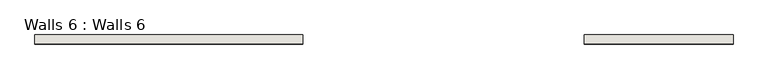
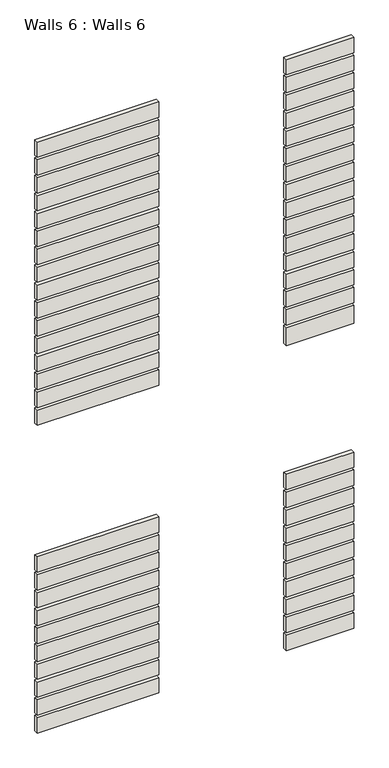
"""IFC4 building model written with IfcOpenShell, lengths in millimetres: wall geometry, Walls 6 : Walls 6."""

from ifc_helpers import new_model, si_unit, frame, origin, place, context, project, spatial, polyline, outline, extrude, source, transform, mapped, element, save


def walls_6_walls_6_f5cc7341(model_context):
    return source(origin(), model_context, "Body", "SweptSolid", [
        extrude(outline(polyline([(142.6430349, 349.9055142), (-2143.3569651, 349.9055142), (-2143.3569651, 426.1055142), (142.6430349, 426.1055142), (142.6430349, 349.9055142)])), frame((0.0, 0.0, 14224.0), z_axis=(0.0, 0.0, 1.0), x_axis=(1.0, 0.0, 0.0)), (0.0, 0.0, 1.0), 304.8),
        extrude(outline(polyline([(142.6430349, 349.9055142), (-2143.3569651, 349.9055142), (-2143.3569651, 426.1055142), (142.6430349, 426.1055142), (142.6430349, 349.9055142)])), frame((0.0, 0.0, 13868.4), z_axis=(0.0, 0.0, 1.0), x_axis=(1.0, 0.0, 0.0)), (0.0, 0.0, 1.0), 304.8),
        extrude(outline(polyline([(142.6430349, 349.9055142), (-2143.3569651, 349.9055142), (-2143.3569651, 426.1055142), (142.6430349, 426.1055142), (142.6430349, 349.9055142)])), frame((0.0, 0.0, 13512.8), z_axis=(0.0, 0.0, 1.0), x_axis=(1.0, 0.0, 0.0)), (0.0, 0.0, 1.0), 304.8),
        extrude(outline(polyline([(142.6430349, 349.9055142), (-2143.3569651, 349.9055142), (-2143.3569651, 426.1055142), (142.6430349, 426.1055142), (142.6430349, 349.9055142)])), frame((0.0, 0.0, 13157.2), z_axis=(0.0, 0.0, 1.0), x_axis=(1.0, 0.0, 0.0)), (0.0, 0.0, 1.0), 304.8),
        extrude(outline(polyline([(142.6430349, 349.9055142), (-2143.3569651, 349.9055142), (-2143.3569651, 426.1055142), (142.6430349, 426.1055142), (142.6430349, 349.9055142)])), frame((0.0, 0.0, 12801.6), z_axis=(0.0, 0.0, 1.0), x_axis=(1.0, 0.0, 0.0)), (0.0, 0.0, 1.0), 304.8),
        extrude(outline(polyline([(142.6430349, 349.9055142), (-2143.3569651, 349.9055142), (-2143.3569651, 426.1055142), (142.6430349, 426.1055142), (142.6430349, 349.9055142)])), frame((0.0, 0.0, 12446.0), z_axis=(0.0, 0.0, 1.0), x_axis=(1.0, 0.0, 0.0)), (0.0, 0.0, 1.0), 304.8),
        extrude(outline(polyline([(142.6430349, 349.9055142), (-2143.3569651, 349.9055142), (-2143.3569651, 426.1055142), (142.6430349, 426.1055142), (142.6430349, 349.9055142)])), frame((0.0, 0.0, 12090.4), z_axis=(0.0, 0.0, 1.0), x_axis=(1.0, 0.0, 0.0)), (0.0, 0.0, 1.0), 304.8),
        extrude(outline(polyline([(142.6430349, 349.9055142), (-2143.3569651, 349.9055142), (-2143.3569651, 426.1055142), (142.6430349, 426.1055142), (142.6430349, 349.9055142)])), frame((0.0, 0.0, 11734.8), z_axis=(0.0, 0.0, 1.0), x_axis=(1.0, 0.0, 0.0)), (0.0, 0.0, 1.0), 304.8),
        extrude(outline(polyline([(142.6430349, 349.9055142), (-2143.3569651, 349.9055142), (-2143.3569651, 426.1055142), (142.6430349, 426.1055142), (142.6430349, 349.9055142)])), frame((0.0, 0.0, 11379.2), z_axis=(0.0, 0.0, 1.0), x_axis=(1.0, 0.0, 0.0)), (0.0, 0.0, 1.0), 304.8),
        extrude(outline(polyline([(142.6430349, 349.9055142), (-2143.3569651, 349.9055142), (-2143.3569651, 426.1055142), (142.6430349, 426.1055142), (142.6430349, 349.9055142)])), frame((0.0, 0.0, 11023.6), z_axis=(0.0, 0.0, 1.0), x_axis=(1.0, 0.0, 0.0)), (0.0, 0.0, 1.0), 304.8),
        extrude(outline(polyline([(142.6430349, 349.9055142), (-2143.3569651, 349.9055142), (-2143.3569651, 426.1055142), (142.6430349, 426.1055142), (142.6430349, 349.9055142)])), frame((0.0, 0.0, 10668.0), z_axis=(0.0, 0.0, 1.0), x_axis=(1.0, 0.0, 0.0)), (0.0, 0.0, 1.0), 304.8),
        extrude(outline(polyline([(142.6430349, 349.9055142), (-2143.3569651, 349.9055142), (-2143.3569651, 426.1055142), (142.6430349, 426.1055142), (142.6430349, 349.9055142)])), frame((0.0, 0.0, 10312.4), z_axis=(0.0, 0.0, 1.0), x_axis=(1.0, 0.0, 0.0)), (0.0, 0.0, 1.0), 304.8),
        extrude(outline(polyline([(142.6430349, 349.9055142), (-2143.3569651, 349.9055142), (-2143.3569651, 426.1055142), (142.6430349, 426.1055142), (142.6430349, 349.9055142)])), frame((0.0, 0.0, 9956.8), z_axis=(0.0, 0.0, 1.0), x_axis=(1.0, 0.0, 0.0)), (0.0, 0.0, 1.0), 304.8),
        extrude(outline(polyline([(142.6430349, 349.9055142), (-2143.3569651, 349.9055142), (-2143.3569651, 426.1055142), (142.6430349, 426.1055142), (142.6430349, 349.9055142)])), frame((0.0, 0.0, 9601.2), z_axis=(0.0, 0.0, 1.0), x_axis=(1.0, 0.0, 0.0)), (0.0, 0.0, 1.0), 304.8),
        extrude(outline(polyline([(142.6430349, 349.9055142), (-2143.3569651, 349.9055142), (-2143.3569651, 426.1055142), (142.6430349, 426.1055142), (142.6430349, 349.9055142)])), frame((0.0, 0.0, 9245.6), z_axis=(0.0, 0.0, 1.0), x_axis=(1.0, 0.0, 0.0)), (0.0, 0.0, 1.0), 304.8),
        extrude(outline(polyline([(142.6430349, 349.9055142), (-2143.3569651, 349.9055142), (-2143.3569651, 426.1055142), (142.6430349, 426.1055142), (142.6430349, 349.9055142)])), frame((0.0, 0.0, 8890.0), z_axis=(0.0, 0.0, 1.0), x_axis=(1.0, 0.0, 0.0)), (0.0, 0.0, 1.0), 304.8),
        extrude(outline(polyline([(142.6430349, 349.9055142), (-2143.3569651, 349.9055142), (-2143.3569651, 426.1055142), (142.6430349, 426.1055142), (142.6430349, 349.9055142)])), frame((0.0, 0.0, 2768.6), z_axis=(0.0, 0.0, 1.0), x_axis=(1.0, 0.0, 0.0)), (0.0, 0.0, 1.0), 304.8),
        extrude(outline(polyline([(3812.9430349, 349.9055142), (2542.9430349, 349.9055142), (2542.9430349, 426.1055142), (3812.9430349, 426.1055142), (3812.9430349, 349.9055142)])), frame((0.0, 0.0, 2768.6), z_axis=(0.0, 0.0, 1.0), x_axis=(1.0, 0.0, 0.0)), (0.0, 0.0, 1.0), 304.8),
        extrude(outline(polyline([(142.6430349, 349.9055142), (-2143.3569651, 349.9055142), (-2143.3569651, 426.1055142), (142.6430349, 426.1055142), (142.6430349, 349.9055142)])), frame((0.0, 0.0, 3124.2), z_axis=(0.0, 0.0, 1.0), x_axis=(1.0, 0.0, 0.0)), (0.0, 0.0, 1.0), 304.8),
        extrude(outline(polyline([(142.6430349, 349.9055142), (-2143.3569651, 349.9055142), (-2143.3569651, 426.1055142), (142.6430349, 426.1055142), (142.6430349, 349.9055142)])), frame((0.0, 0.0, 3479.8), z_axis=(0.0, 0.0, 1.0), x_axis=(1.0, 0.0, 0.0)), (0.0, 0.0, 1.0), 304.8),
        extrude(outline(polyline([(142.6430349, 349.9055142), (-2143.3569651, 349.9055142), (-2143.3569651, 426.1055142), (142.6430349, 426.1055142), (142.6430349, 349.9055142)])), frame((0.0, 0.0, 3835.4), z_axis=(0.0, 0.0, 1.0), x_axis=(1.0, 0.0, 0.0)), (0.0, 0.0, 1.0), 304.8),
        extrude(outline(polyline([(142.6430349, 349.9055142), (-2143.3569651, 349.9055142), (-2143.3569651, 426.1055142), (142.6430349, 426.1055142), (142.6430349, 349.9055142)])), frame((0.0, 0.0, 4191.0), z_axis=(0.0, 0.0, 1.0), x_axis=(1.0, 0.0, 0.0)), (0.0, 0.0, 1.0), 304.8),
        extrude(outline(polyline([(142.6430349, 349.9055142), (-2143.3569651, 349.9055142), (-2143.3569651, 426.1055142), (142.6430349, 426.1055142), (142.6430349, 349.9055142)])), frame((0.0, 0.0, 4546.6), z_axis=(0.0, 0.0, 1.0), x_axis=(1.0, 0.0, 0.0)), (0.0, 0.0, 1.0), 304.8),
        extrude(outline(polyline([(142.6430349, 349.9055142), (-2143.3569651, 349.9055142), (-2143.3569651, 426.1055142), (142.6430349, 426.1055142), (142.6430349, 349.9055142)])), frame((0.0, 0.0, 4902.2), z_axis=(0.0, 0.0, 1.0), x_axis=(1.0, 0.0, 0.0)), (0.0, 0.0, 1.0), 304.8),
        extrude(outline(polyline([(142.6430349, 349.9055142), (-2143.3569651, 349.9055142), (-2143.3569651, 426.1055142), (142.6430349, 426.1055142), (142.6430349, 349.9055142)])), frame((0.0, 0.0, 5257.8), z_axis=(0.0, 0.0, 1.0), x_axis=(1.0, 0.0, 0.0)), (0.0, 0.0, 1.0), 304.8),
        extrude(outline(polyline([(142.6430349, 349.9055142), (-2143.3569651, 349.9055142), (-2143.3569651, 426.1055142), (142.6430349, 426.1055142), (142.6430349, 349.9055142)])), frame((0.0, 0.0, 5613.4), z_axis=(0.0, 0.0, 1.0), x_axis=(1.0, 0.0, 0.0)), (0.0, 0.0, 1.0), 304.8),
        extrude(outline(polyline([(142.6430349, 349.9055142), (-2143.3569651, 349.9055142), (-2143.3569651, 426.1055142), (142.6430349, 426.1055142), (142.6430349, 349.9055142)])), frame((0.0, 0.0, 5969.0), z_axis=(0.0, 0.0, 1.0), x_axis=(1.0, 0.0, 0.0)), (0.0, 0.0, 1.0), 304.8),
        extrude(outline(polyline([(3812.9430349, 349.9055142), (2542.9430349, 349.9055142), (2542.9430349, 426.1055142), (3812.9430349, 426.1055142), (3812.9430349, 349.9055142)])), frame((0.0, 0.0, 3124.2), z_axis=(0.0, 0.0, 1.0), x_axis=(1.0, 0.0, 0.0)), (0.0, 0.0, 1.0), 304.8),
        extrude(outline(polyline([(3812.9430349, 349.9055142), (2542.9430349, 349.9055142), (2542.9430349, 426.1055142), (3812.9430349, 426.1055142), (3812.9430349, 349.9055142)])), frame((0.0, 0.0, 3479.8), z_axis=(0.0, 0.0, 1.0), x_axis=(1.0, 0.0, 0.0)), (0.0, 0.0, 1.0), 304.8),
        extrude(outline(polyline([(3812.9430349, 349.9055142), (2542.9430349, 349.9055142), (2542.9430349, 426.1055142), (3812.9430349, 426.1055142), (3812.9430349, 349.9055142)])), frame((0.0, 0.0, 3835.4), z_axis=(0.0, 0.0, 1.0), x_axis=(1.0, 0.0, 0.0)), (0.0, 0.0, 1.0), 304.8),
        extrude(outline(polyline([(3812.9430349, 349.9055142), (2542.9430349, 349.9055142), (2542.9430349, 426.1055142), (3812.9430349, 426.1055142), (3812.9430349, 349.9055142)])), frame((0.0, 0.0, 4191.0), z_axis=(0.0, 0.0, 1.0), x_axis=(1.0, 0.0, 0.0)), (0.0, 0.0, 1.0), 304.8),
        extrude(outline(polyline([(3812.9430349, 349.9055142), (2542.9430349, 349.9055142), (2542.9430349, 426.1055142), (3812.9430349, 426.1055142), (3812.9430349, 349.9055142)])), frame((0.0, 0.0, 4546.6), z_axis=(0.0, 0.0, 1.0), x_axis=(1.0, 0.0, 0.0)), (0.0, 0.0, 1.0), 304.8),
        extrude(outline(polyline([(3812.9430349, 349.9055142), (2542.9430349, 349.9055142), (2542.9430349, 426.1055142), (3812.9430349, 426.1055142), (3812.9430349, 349.9055142)])), frame((0.0, 0.0, 4902.2), z_axis=(0.0, 0.0, 1.0), x_axis=(1.0, 0.0, 0.0)), (0.0, 0.0, 1.0), 304.8),
        extrude(outline(polyline([(3812.9430349, 349.9055142), (2542.9430349, 349.9055142), (2542.9430349, 426.1055142), (3812.9430349, 426.1055142), (3812.9430349, 349.9055142)])), frame((0.0, 0.0, 5257.8), z_axis=(0.0, 0.0, 1.0), x_axis=(1.0, 0.0, 0.0)), (0.0, 0.0, 1.0), 304.8),
        extrude(outline(polyline([(3812.9430349, 349.9055142), (2542.9430349, 349.9055142), (2542.9430349, 426.1055142), (3812.9430349, 426.1055142), (3812.9430349, 349.9055142)])), frame((0.0, 0.0, 5613.4), z_axis=(0.0, 0.0, 1.0), x_axis=(1.0, 0.0, 0.0)), (0.0, 0.0, 1.0), 304.8),
        extrude(outline(polyline([(3812.9430349, 349.9055142), (2542.9430349, 349.9055142), (2542.9430349, 426.1055142), (3812.9430349, 426.1055142), (3812.9430349, 349.9055142)])), frame((0.0, 0.0, 5969.0), z_axis=(0.0, 0.0, 1.0), x_axis=(1.0, 0.0, 0.0)), (0.0, 0.0, 1.0), 304.8),
        extrude(outline(polyline([(3812.9430349, 349.9055142), (2542.9430349, 349.9055142), (2542.9430349, 426.1055142), (3812.9430349, 426.1055142), (3812.9430349, 349.9055142)])), frame((0.0, 0.0, 8835.326551), z_axis=(0.0, 0.0, 1.0), x_axis=(1.0, 0.0, 0.0)), (0.0, 0.0, 1.0), 359.473449),
        extrude(outline(polyline([(3812.9430349, 349.9055142), (2542.9430349, 349.9055142), (2542.9430349, 426.1055142), (3812.9430349, 426.1055142), (3812.9430349, 349.9055142)])), frame((0.0, 0.0, 9245.6), z_axis=(0.0, 0.0, 1.0), x_axis=(1.0, 0.0, 0.0)), (0.0, 0.0, 1.0), 304.8),
        extrude(outline(polyline([(3812.9430349, 349.9055142), (2542.9430349, 349.9055142), (2542.9430349, 426.1055142), (3812.9430349, 426.1055142), (3812.9430349, 349.9055142)])), frame((0.0, 0.0, 9601.2), z_axis=(0.0, 0.0, 1.0), x_axis=(1.0, 0.0, 0.0)), (0.0, 0.0, 1.0), 304.8),
        extrude(outline(polyline([(3812.9430349, 349.9055142), (2542.9430349, 349.9055142), (2542.9430349, 426.1055142), (3812.9430349, 426.1055142), (3812.9430349, 349.9055142)])), frame((0.0, 0.0, 9956.8), z_axis=(0.0, 0.0, 1.0), x_axis=(1.0, 0.0, 0.0)), (0.0, 0.0, 1.0), 304.8),
        extrude(outline(polyline([(3812.9430349, 349.9055142), (2542.9430349, 349.9055142), (2542.9430349, 426.1055142), (3812.9430349, 426.1055142), (3812.9430349, 349.9055142)])), frame((0.0, 0.0, 10312.4), z_axis=(0.0, 0.0, 1.0), x_axis=(1.0, 0.0, 0.0)), (0.0, 0.0, 1.0), 304.8),
        extrude(outline(polyline([(3812.9430349, 349.9055142), (2542.9430349, 349.9055142), (2542.9430349, 426.1055142), (3812.9430349, 426.1055142), (3812.9430349, 349.9055142)])), frame((0.0, 0.0, 10668.0), z_axis=(0.0, 0.0, 1.0), x_axis=(1.0, 0.0, 0.0)), (0.0, 0.0, 1.0), 304.8),
        extrude(outline(polyline([(3812.9430349, 349.9055142), (2542.9430349, 349.9055142), (2542.9430349, 426.1055142), (3812.9430349, 426.1055142), (3812.9430349, 349.9055142)])), frame((0.0, 0.0, 11023.6), z_axis=(0.0, 0.0, 1.0), x_axis=(1.0, 0.0, 0.0)), (0.0, 0.0, 1.0), 304.8),
        extrude(outline(polyline([(3812.9430349, 349.9055142), (2542.9430349, 349.9055142), (2542.9430349, 426.1055142), (3812.9430349, 426.1055142), (3812.9430349, 349.9055142)])), frame((0.0, 0.0, 11379.2), z_axis=(0.0, 0.0, 1.0), x_axis=(1.0, 0.0, 0.0)), (0.0, 0.0, 1.0), 304.8),
        extrude(outline(polyline([(3812.9430349, 349.9055142), (2542.9430349, 349.9055142), (2542.9430349, 426.1055142), (3812.9430349, 426.1055142), (3812.9430349, 349.9055142)])), frame((0.0, 0.0, 11734.8), z_axis=(0.0, 0.0, 1.0), x_axis=(1.0, 0.0, 0.0)), (0.0, 0.0, 1.0), 304.8),
        extrude(outline(polyline([(3812.9430349, 349.9055142), (2542.9430349, 349.9055142), (2542.9430349, 426.1055142), (3812.9430349, 426.1055142), (3812.9430349, 349.9055142)])), frame((0.0, 0.0, 12090.4), z_axis=(0.0, 0.0, 1.0), x_axis=(1.0, 0.0, 0.0)), (0.0, 0.0, 1.0), 304.8),
        extrude(outline(polyline([(3812.9430349, 349.9055142), (2542.9430349, 349.9055142), (2542.9430349, 426.1055142), (3812.9430349, 426.1055142), (3812.9430349, 349.9055142)])), frame((0.0, 0.0, 12446.0), z_axis=(0.0, 0.0, 1.0), x_axis=(1.0, 0.0, 0.0)), (0.0, 0.0, 1.0), 304.8),
        extrude(outline(polyline([(3812.9430349, 349.9055142), (2542.9430349, 349.9055142), (2542.9430349, 426.1055142), (3812.9430349, 426.1055142), (3812.9430349, 349.9055142)])), frame((0.0, 0.0, 12801.6), z_axis=(0.0, 0.0, 1.0), x_axis=(1.0, 0.0, 0.0)), (0.0, 0.0, 1.0), 304.8),
        extrude(outline(polyline([(3812.9430349, 349.9055142), (2542.9430349, 349.9055142), (2542.9430349, 426.1055142), (3812.9430349, 426.1055142), (3812.9430349, 349.9055142)])), frame((0.0, 0.0, 13157.2), z_axis=(0.0, 0.0, 1.0), x_axis=(1.0, 0.0, 0.0)), (0.0, 0.0, 1.0), 304.8),
        extrude(outline(polyline([(3812.9430349, 349.9055142), (2542.9430349, 349.9055142), (2542.9430349, 426.1055142), (3812.9430349, 426.1055142), (3812.9430349, 349.9055142)])), frame((0.0, 0.0, 13512.8), z_axis=(0.0, 0.0, 1.0), x_axis=(1.0, 0.0, 0.0)), (0.0, 0.0, 1.0), 304.8),
        extrude(outline(polyline([(3812.9430349, 349.9055142), (2542.9430349, 349.9055142), (2542.9430349, 426.1055142), (3812.9430349, 426.1055142), (3812.9430349, 349.9055142)])), frame((0.0, 0.0, 13868.4), z_axis=(0.0, 0.0, 1.0), x_axis=(1.0, 0.0, 0.0)), (0.0, 0.0, 1.0), 304.8),
        extrude(outline(polyline([(3812.9430349, 349.9055142), (2542.9430349, 349.9055142), (2542.9430349, 426.1055142), (3812.9430349, 426.1055142), (3812.9430349, 349.9055142)])), frame((0.0, 0.0, 14224.0), z_axis=(0.0, 0.0, 1.0), x_axis=(1.0, 0.0, 0.0)), (0.0, 0.0, 1.0), 304.8),
    ])


if __name__ == "__main__":
    model = new_model("IFC4")
    model_context = context("Model", 3, world=origin())
    ifc_project = project(units=[si_unit("LENGTHUNIT", "METRE", prefix="MILLI")], contexts=[model_context])
    site = spatial("IfcSite", under=ifc_project)
    building = spatial("IfcBuilding", under=site)
    placement = place(None, origin())
    walls_6_walls_6_shape = walls_6_walls_6_f5cc7341(model_context)
    element("IfcWall", 1, ObjectType="Walls 6 : Walls 6", at=placement, inside=building, context=model_context, shape_type="MappedRepresentation", body=[
        mapped(walls_6_walls_6_shape, transform((0.0, 0.0, 0.0), x_axis=(1.0, 0.0, 0.0), y_axis=(0.0, 1.0, 0.0), z_axis=(0.0, 0.0, 1.0))),
    ])
    save(model, "model.ifc")

# Revit data of these elements
# Element 1 (IfcWall, "Walls 6 : Walls 6")
#   Materials on its faces: "Default Wall", "1 wood"
# Materials
#   "Default Wall": colour RGB 128 128 128, transparency 0, Cost = 0
#   "1 wood": class "Generic", colour RGB 120 120 120, transparency 0, Cost = 0
